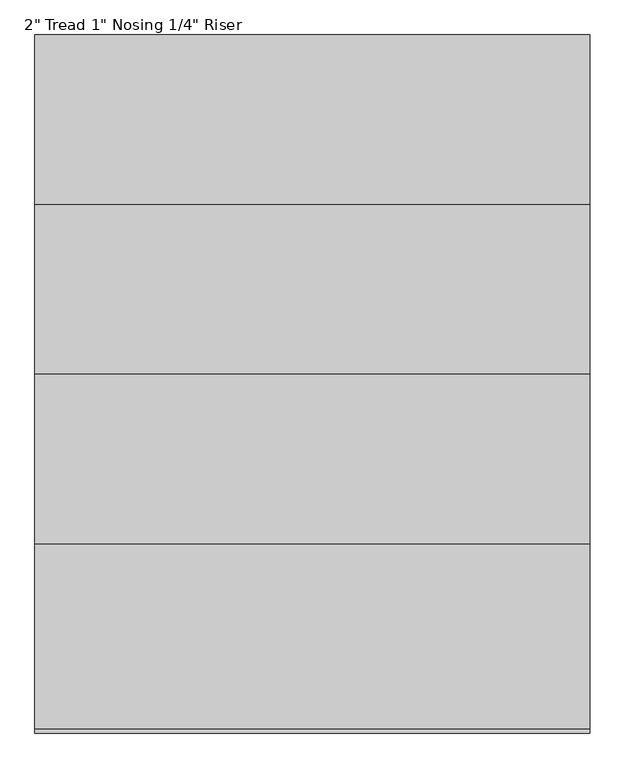
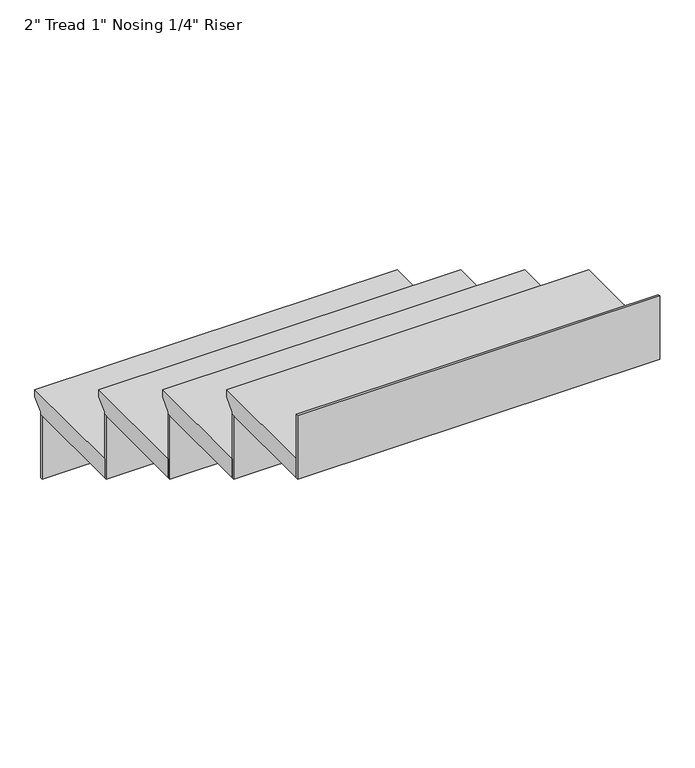
"""IFC4 building model written with IfcOpenShell, lengths in millimetres: stair flight geometry."""

from ifc_helpers import new_model, si_unit, frame, origin, place, context, project, spatial, polyline, outline, extrude, source, transform, mapped, element, save


def stair_flight_4ac50f61(model_context):
    return source(origin(), model_context, "Body", "SweptSolid", [
        extrude(outline(polyline([(22889.9216096, 33701.2839133), (23194.7216096, 33701.2839133), (23194.7216096, 33682.2339133), (23169.3216096, 33656.8339133), (23169.3216096, 33650.4839133), (22889.9216096, 33650.4839133), (22889.9216096, 33701.2839133)])), frame((-2398.2415084, 0.0, 0.0), z_axis=(1.0, 0.0, 0.0), x_axis=(0.0, 1.0, 0.0)), (0.0, 0.0, 1.0), 914.4),
        extrude(outline(polyline([(-2398.2415084, 23162.9716096), (-2398.2415084, 23169.3216096), (-1483.8415084, 23169.3216096), (-1483.8415084, 23162.9716096), (-2398.2415084, 23162.9716096)])), frame((0.0, 0.0, 33481.1505799), z_axis=(0.0, 0.0, 1.0), x_axis=(1.0, 0.0, 0.0)), (0.0, 0.0, 1.0), 169.3333333),
        extrude(outline(polyline([(-2398.2415084, 22883.5716096), (-2398.2415084, 22889.9216096), (-1483.8415084, 22889.9216096), (-1483.8415084, 22883.5716096), (-2398.2415084, 22883.5716096)])), frame((0.0, 0.0, 33650.4839133), z_axis=(0.0, 0.0, 1.0), x_axis=(1.0, 0.0, 0.0)), (0.0, 0.0, 1.0), 169.3333333),
        extrude(outline(polyline([(22610.5216096, 33870.6172466), (22915.3216096, 33870.6172466), (22915.3216096, 33851.5672466), (22889.9216096, 33826.1672466), (22889.9216096, 33819.8172466), (22610.5216096, 33819.8172466), (22610.5216096, 33870.6172466)])), frame((-2398.2415084, 0.0, 0.0), z_axis=(1.0, 0.0, 0.0), x_axis=(0.0, 1.0, 0.0)), (0.0, 0.0, 1.0), 914.4),
        extrude(outline(polyline([(-2398.2415084, 22604.1716096), (-2398.2415084, 22610.5216096), (-1483.8415084, 22610.5216096), (-1483.8415084, 22604.1716096), (-2398.2415084, 22604.1716096)])), frame((0.0, 0.0, 33819.8172466), z_axis=(0.0, 0.0, 1.0), x_axis=(1.0, 0.0, 0.0)), (0.0, 0.0, 1.0), 169.3333333),
        extrude(outline(polyline([(22331.1216096, 34039.9505799), (22635.9216096, 34039.9505799), (22635.9216096, 34020.9005799), (22610.5216096, 33995.5005799), (22610.5216096, 33989.1505799), (22331.1216096, 33989.1505799), (22331.1216096, 34039.9505799)])), frame((-2398.2415084, 0.0, 0.0), z_axis=(1.0, 0.0, 0.0), x_axis=(0.0, 1.0, 0.0)), (0.0, 0.0, 1.0), 914.4),
        extrude(outline(polyline([(-2398.2415084, 22324.7716096), (-2398.2415084, 22331.1216096), (-1483.8415084, 22331.1216096), (-1483.8415084, 22324.7716096), (-2398.2415084, 22324.7716096)])), frame((0.0, 0.0, 33989.1505799), z_axis=(0.0, 0.0, 1.0), x_axis=(1.0, 0.0, 0.0)), (0.0, 0.0, 1.0), 169.3333333),
        extrude(outline(polyline([(-2398.2415084, 22045.3716096), (-2398.2415084, 22051.7216096), (-1483.8415084, 22051.7216096), (-1483.8415084, 22045.3716096), (-2398.2415084, 22045.3716096)])), frame((0.0, 0.0, 34158.4839133), z_axis=(0.0, 0.0, 1.0), x_axis=(1.0, 0.0, 0.0)), (0.0, 0.0, 1.0), 169.3333333),
        extrude(outline(polyline([(22051.7216096, 34209.2839133), (22356.5216096, 34209.2839133), (22356.5216096, 34190.2339133), (22331.1216096, 34164.8339133), (22331.1216096, 34158.4839133), (22051.7216096, 34158.4839133), (22051.7216096, 34209.2839133)])), frame((-2398.2415084, 0.0, 0.0), z_axis=(1.0, 0.0, 0.0), x_axis=(0.0, 1.0, 0.0)), (0.0, 0.0, 1.0), 914.4),
    ])


if __name__ == "__main__":
    model = new_model("IFC4")
    model_context = context("Model", 3, world=origin())
    ifc_project = project(units=[si_unit("LENGTHUNIT", "METRE", prefix="MILLI")], contexts=[model_context])
    site = spatial("IfcSite", under=ifc_project)
    building = spatial("IfcBuilding", under=site)
    placement = place(None, origin())
    stair_flight_shape = stair_flight_4ac50f61(model_context)
    element("IfcStairFlight", 1, ObjectType="2\" Tread 1\" Nosing 1/4\" Riser", at=placement, inside=building, context=model_context, shape_type="MappedRepresentation", body=[
        mapped(stair_flight_shape, transform((0.0, 0.0, 0.0), x_axis=(1.0, 0.0, 0.0), y_axis=(0.0, 1.0, 0.0), z_axis=(0.0, 0.0, 1.0))),
    ])
    save(model, "model.ifc")
